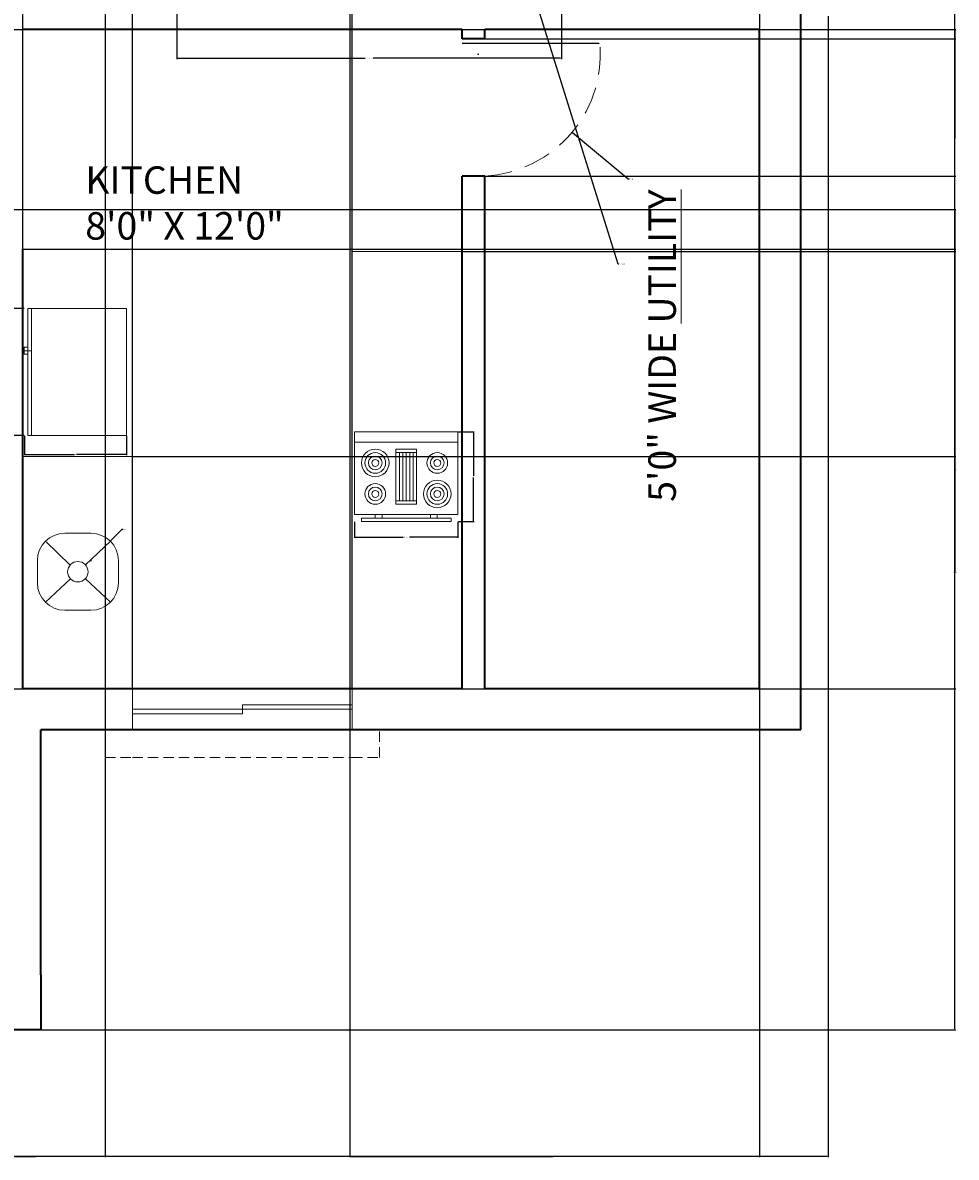
# Model space of a CAD drawing. Units: inches. Extents: x 6662 to 7211, y 5077 to 5683.
# Tile 4 of 9: x 7007 to 7211, y 5077 to 5325. Entities that reach past the tile are written whole.
import ezdxf

# ---------------------------------------------------------------- set-up
doc = ezdxf.new("R2010")
doc.units = ezdxf.units.IN
doc.header["$LTSCALE"] = 3
doc.header["$MEASUREMENT"] = 0
doc.linetypes.add('HIDDEN', pattern=[0.375, 0.25, -0.125])
for name, color, linetype, lineweight in [('A-ANNO-DIMS', 2, 'Continuous', 18), ('A-AREA-IDEN', 7, 'Continuous', 18), ('A-DOOR', 4, 'Continuous', 25), ('A-DOOR-HIDN', 4, 'HIDDEN', 13), ('A-EQPM', 8, 'Continuous', 18), ('A-FLOR-CASE', 8, 'Continuous', 20), ('A-FLOR-CASE-PATT', 241, 'Continuous', 13), ('A-FLOR-FIXT', 8, 'Continuous', 18), ('A-GLAZ', 4, 'Continuous', 18), ('A-GLAZ-OVHD', 4, 'HIDDEN', 13), ('A-WALL', 7, 'Continuous', 35)]:
    doc.layers.add(name, color=color, linetype=linetype, lineweight=lineweight)
doc.styles.get("Standard").update_dxf_attribs({"font": 'arial.ttf'})
doc.dimstyles.get("Standard").update_dxf_attribs({"dimtxt": 0.18, "dimasz": 0.18, "dimexe": 0.18, "dimexo": 0.0625, "dimgap": 0.09, "dimtad": 0, "dimtih": 1, "dimtoh": 1, "dimdec": 4, "dimzin": 0, "dimdsep": 46, "dimtxsty": 'Standard', "dimcen": 0.09, "dimadec": 0, "dimazin": 0, "dimtfac": 1, "dimtdec": 4, "dimtofl": 0, "dimtmove": 0, "dimatfit": 3, "dimfxl": 1, "dimtolj": 1, "dimtzin": 0, "dimarcsym": 0})

# ---------------------------------------------------------------- blocks, each defined once
blk = doc.blocks.new('Range-Oven - 30 in top')
for p, q in [((0, -3), (30, -3)), ((12, -6), (18, -6)), ((13, -20), (13, -6)), ((14, -6), (14, -20)), ((15, -20), (15, -6)), ((16, -6), (16, -20)), ((17, -20), (17, -6)), ((18, -20), (12, -20)), ((6, -24), (6, -25)), ((8, -25), (8, -24)), ((22, -25), (22, -24)), ((24, -24), (24, -25))]:
    blk.add_line(p, q)
for points in [[(0, -24), (0, 0), (30, 0), (30, -24)], [(12, -21), (12, -5), (18, -5), (18, -21)], [(2, -26), (2, -25), (28, -25), (28, -26)]]:
    blk.add_lwpolyline(points, close=True)
for centre, radius in [((6, -9), 4), ((6, -9), 3), ((24, -9), 3), ((6, -9), 2), ((6, -9), 1), ((24, -9), 2), ((24, -9), 1), ((6, -18), 3), ((6, -18), 2), ((24, -18), 4), ((24, -18), 3), ((24, -18), 2), ((6, -18), 1), ((24, -18), 1)]:
    blk.add_circle(centre, radius)
blk = doc.blocks.new('Refrigerator-2 door - 36 in top')
for p, q in [((0, -26.999999), (36, -26.999999)), ((11, -27.999999), (11, -28.999999)), ((12, -26.999999), (12, -28.999999)), ((13, -28.999999), (13, -27.999999)), ((11, -28.999999), (13, -28.999999))]:
    blk.add_line(p, q)
blk.add_lwpolyline([(0, -27.999999), (0, 0), (36, 0), (36, -27.999999)], close=True)
blk = doc.blocks.new('*D28')
at = {"layer": 'A-ANNO-DIMS', "color": 0, "lineweight": -2, "ltscale": 3, "transparency": 16777216}
for p, q in [((7040.57, 5329.37), (7040.57, 5316.65)), ((7124.57, 5329.37), (7124.57, 5316.65)), ((7040.75, 5316.83), (7081.66, 5316.83)), ((7124.39, 5316.83), (7083.47, 5316.83))]:
    blk.add_line(p, q, dxfattribs=at)
at = {"layer": 'A-ANNO-DIMS', "color": 0, "ltscale": 3, "transparency": 16777216}
for points in [[(7040.75, 5316.86), (7040.75, 5316.8), (7040.57, 5316.83)], [(7124.39, 5316.86), (7124.39, 5316.8), (7124.57, 5316.83)]]:
    blk.add_solid(points, dxfattribs=at)
at = {"layer": 'Defpoints', "color": 0, "ltscale": 3, "transparency": 16777216}
for p in [(7040.57, 5329.43), (7124.57, 5329.43), (7040.57, 5316.83)]:
    blk.add_point(p, dxfattribs=at)
at = {"layer": 'A-ANNO-DIMS', "color": 0, "ltscale": 3, "transparency": 16777216, "insert": (7082.57, 5316.83), "char_height": 0.18, "attachment_point": 5}
blk.add_mtext('\\A1;SOFA 84 TYP.', dxfattribs=at)
blk = doc.blocks.new('*D34')
at = {"layer": 'A-ANNO-DIMS', "color": 0, "lineweight": -2, "ltscale": 3, "transparency": 16777216}
for p, q in [((7079.39, 5215.56), (7079.39, 5212.05)), ((7101.96, 5215.56), (7101.96, 5212.05)), ((7079.57, 5212.23), (7089.98, 5212.23)), ((7101.78, 5212.23), (7091.37, 5212.23))]:
    blk.add_line(p, q, dxfattribs=at)
at = {"layer": 'A-ANNO-DIMS', "color": 0, "ltscale": 3, "transparency": 16777216}
for points in [[(7079.57, 5212.26), (7079.57, 5212.2), (7079.39, 5212.23)], [(7101.78, 5212.26), (7101.78, 5212.2), (7101.96, 5212.23)]]:
    blk.add_solid(points, dxfattribs=at)
at = {"layer": 'Defpoints', "color": 0, "ltscale": 3, "transparency": 16777216}
for p in [(7079.39, 5215.62), (7101.96, 5215.62), (7101.96, 5212.23)]:
    blk.add_point(p, dxfattribs=at)
at = {"layer": 'A-ANNO-DIMS', "color": 0, "ltscale": 3, "transparency": 16777216, "insert": (7090.67, 5212.23), "char_height": 0.18, "attachment_point": 5}
blk.add_mtext('\\A1;RANGE 23', dxfattribs=at)
blk = doc.blocks.new('*D35')
at = {"layer": 'A-ANNO-DIMS', "color": 0, "lineweight": -2, "ltscale": 3, "transparency": 16777216}
for p, q in [((7102.02, 5235.18), (7105.53, 5235.18)), ((7105.35, 5235), (7105.35, 5225.58)), ((7105.35, 5215.8), (7105.35, 5225.22)), ((7102.02, 5215.62), (7105.53, 5215.62))]:
    blk.add_line(p, q, dxfattribs=at)
at = {"layer": 'A-ANNO-DIMS', "color": 0, "ltscale": 3, "transparency": 16777216}
for points in [[(7105.32, 5235), (7105.38, 5235), (7105.35, 5235.18)], [(7105.32, 5215.8), (7105.38, 5215.8), (7105.35, 5215.62)]]:
    blk.add_solid(points, dxfattribs=at)
at = {"layer": 'Defpoints', "color": 0, "ltscale": 3, "transparency": 16777216}
for p in [(7101.96, 5235.18), (7105.35, 5235.18), (7101.96, 5215.62)]:
    blk.add_point(p, dxfattribs=at)
at = {"layer": 'A-ANNO-DIMS', "color": 0, "ltscale": 3, "transparency": 16777216, "insert": (7105.35, 5225.4), "char_height": 0.18, "attachment_point": 5}
blk.add_mtext('\\A1;20', dxfattribs=at)
blk = doc.blocks.new('*D36')
at = {"layer": 'A-ANNO-DIMS', "color": 0, "lineweight": -2, "ltscale": 3, "transparency": 16777216}
for p, q in [((7007.15, 5262.16), (7002.88, 5262.16)), ((7003.06, 5261.98), (7003.06, 5248.48)), ((7003.06, 5234.61), (7003.06, 5248.11)), ((7007.15, 5234.43), (7002.88, 5234.43))]:
    blk.add_line(p, q, dxfattribs=at)
at = {"layer": 'A-ANNO-DIMS', "color": 0, "ltscale": 3, "transparency": 16777216}
for points in [[(7003.03, 5261.98), (7003.09, 5261.98), (7003.06, 5262.16)], [(7003.03, 5234.61), (7003.09, 5234.61), (7003.06, 5234.43)]]:
    blk.add_solid(points, dxfattribs=at)
at = {"layer": 'Defpoints', "color": 0, "ltscale": 3, "transparency": 16777216}
for p in [(7007.22, 5262.16), (7003.06, 5234.43), (7007.22, 5234.43)]:
    blk.add_point(p, dxfattribs=at)
at = {"layer": 'A-ANNO-DIMS', "color": 0, "ltscale": 3, "transparency": 16777216, "insert": (7003.06, 5248.29), "char_height": 0.18, "attachment_point": 5}
blk.add_mtext('\\A1;REFRIGERATOR 28', dxfattribs=at)
blk = doc.blocks.new('*D37')
at = {"layer": 'A-ANNO-DIMS', "color": 0, "lineweight": -2, "ltscale": 3, "transparency": 16777216}
for p, q in [((7007.22, 5234.37), (7007.22, 5230.09)), ((7029.56, 5234.37), (7029.56, 5230.09)), ((7007.4, 5230.27), (7018.17, 5230.27)), ((7029.38, 5230.27), (7018.61, 5230.27))]:
    blk.add_line(p, q, dxfattribs=at)
at = {"layer": 'A-ANNO-DIMS', "color": 0, "ltscale": 3, "transparency": 16777216}
for points in [[(7007.4, 5230.3), (7007.4, 5230.24), (7007.22, 5230.27)], [(7029.38, 5230.3), (7029.38, 5230.24), (7029.56, 5230.27)]]:
    blk.add_solid(points, dxfattribs=at)
at = {"layer": 'Defpoints', "color": 0, "ltscale": 3, "transparency": 16777216}
for p in [(7007.22, 5234.43), (7029.56, 5234.43), (7029.56, 5230.27)]:
    blk.add_point(p, dxfattribs=at)
at = {"layer": 'A-ANNO-DIMS', "color": 0, "ltscale": 3, "transparency": 16777216, "insert": (7018.39, 5230.27), "char_height": 0.18, "attachment_point": 5}
blk.add_mtext('\\A1;22', dxfattribs=at)
blk = doc.blocks.new('*D40')
at = {"layer": 'A-ANNO-DIMS', "color": 0, "lineweight": -2, "ltscale": 3, "transparency": 16777216}
for p, q in [((7182.86, 5326.04), (7182.86, 5076.72)), ((6689.86, 5323.04), (6689.86, 5076.72)), ((6690.04, 5076.9), (6936.07, 5076.9)), ((7182.68, 5076.9), (6936.65, 5076.9))]:
    blk.add_line(p, q, dxfattribs=at)
at = {"layer": 'A-ANNO-DIMS', "color": 0, "ltscale": 3, "transparency": 16777216}
for points in [[(6690.04, 5076.93), (6690.04, 5076.87), (6689.86, 5076.9)], [(7182.68, 5076.93), (7182.68, 5076.87), (7182.86, 5076.9)]]:
    blk.add_solid(points, dxfattribs=at)
at = {"layer": 'Defpoints', "color": 0, "ltscale": 3, "transparency": 16777216}
for p in [(7182.86, 5326.1), (6689.86, 5323.1), (7182.86, 5076.9)]:
    blk.add_point(p, dxfattribs=at)
at = {"layer": 'A-ANNO-DIMS', "color": 0, "ltscale": 3, "transparency": 16777216, "insert": (6936.36, 5076.9), "char_height": 0.18, "attachment_point": 5}
blk.add_mtext('\\A1;493', dxfattribs=at)
blk = doc.blocks.new('*D41')
at = {"layer": 'A-ANNO-DIMS', "color": 0, "lineweight": -2, "ltscale": 3, "transparency": 16777216}
for p, q in [((7035.92, 5655.02), (7210.74, 5655.02)), ((7210.56, 5654.84), (7210.56, 5379.99)), ((7210.56, 5104.78), (7210.56, 5379.63)), ((7010.92, 5104.6), (7210.74, 5104.6))]:
    blk.add_line(p, q, dxfattribs=at)
at = {"layer": 'A-ANNO-DIMS', "color": 0, "ltscale": 3, "transparency": 16777216}
for points in [[(7210.53, 5654.84), (7210.59, 5654.84), (7210.56, 5655.02)], [(7210.53, 5104.78), (7210.59, 5104.78), (7210.56, 5104.6)]]:
    blk.add_solid(points, dxfattribs=at)
at = {"layer": 'Defpoints', "color": 0, "ltscale": 3, "transparency": 16777216}
for p in [(7035.86, 5655.02), (7210.56, 5655.02), (7010.86, 5104.6)]:
    blk.add_point(p, dxfattribs=at)
at = {"layer": 'A-ANNO-DIMS', "color": 0, "ltscale": 3, "transparency": 16777216, "insert": (7210.56, 5379.81), "char_height": 0.18, "attachment_point": 5}
blk.add_mtext('\\A1;550.4', dxfattribs=at)
blk = doc.blocks.new('*D67')
at = {"layer": 'A-ANNO-DIMS', "color": 0, "lineweight": -2, "ltscale": 3, "transparency": 16777216}
for p, q in [((6994.86, 5514.54), (6994.86, 5076.72)), ((7024.86, 5514.54), (7024.86, 5076.72)), ((6995.04, 5076.9), (7009.64, 5076.9)), ((7024.68, 5076.9), (7010.08, 5076.9))]:
    blk.add_line(p, q, dxfattribs=at)
at = {"layer": 'A-ANNO-DIMS', "color": 0, "ltscale": 3, "transparency": 16777216}
for points in [[(6995.04, 5076.93), (6995.04, 5076.87), (6994.86, 5076.9)], [(7024.68, 5076.93), (7024.68, 5076.87), (7024.86, 5076.9)]]:
    blk.add_solid(points, dxfattribs=at)
at = {"layer": 'Defpoints', "color": 0, "ltscale": 3, "transparency": 16777216}
for p in [(6994.86, 5514.6), (7024.86, 5514.6), (7024.86, 5076.9)]:
    blk.add_point(p, dxfattribs=at)
at = {"layer": 'A-ANNO-DIMS', "color": 0, "ltscale": 3, "transparency": 16777216, "insert": (7009.86, 5076.9), "char_height": 0.18, "attachment_point": 5}
blk.add_mtext('\\A1;30', dxfattribs=at)
blk = doc.blocks.new('*D69')
at = {"layer": 'A-ANNO-DIMS', "color": 0, "lineweight": -2, "ltscale": 3, "transparency": 16777216}
for p, q in [((7107.92, 5321.1), (7210.74, 5321.1)), ((7210.56, 5320.92), (7210.56, 5306.28)), ((7210.56, 5291.28), (7210.56, 5305.92)), ((7107.92, 5291.1), (7210.74, 5291.1))]:
    blk.add_line(p, q, dxfattribs=at)
at = {"layer": 'A-ANNO-DIMS', "color": 0, "ltscale": 3, "transparency": 16777216}
for points in [[(7210.53, 5320.92), (7210.59, 5320.92), (7210.56, 5321.1)], [(7210.53, 5291.28), (7210.59, 5291.28), (7210.56, 5291.1)]]:
    blk.add_solid(points, dxfattribs=at)
at = {"layer": 'Defpoints', "color": 0, "ltscale": 3, "transparency": 16777216}
for p in [(7107.86, 5321.1), (7210.56, 5321.1), (7107.86, 5291.1)]:
    blk.add_point(p, dxfattribs=at)
at = {"layer": 'A-ANNO-DIMS', "color": 0, "ltscale": 3, "transparency": 16777216, "insert": (7210.56, 5306.1), "char_height": 0.18, "attachment_point": 5}
blk.add_mtext('\\A1;30', dxfattribs=at)
blk = doc.blocks.new('*D74')
at = {"layer": 'A-ANNO-DIMS', "color": 0, "lineweight": -2, "ltscale": 3, "transparency": 16777216}
for p, q in [((7006.86, 5179.16), (7006.86, 5682.9)), ((7007.04, 5682.72), (7018.64, 5682.72)), ((7030.68, 5682.72), (7019.08, 5682.72)), ((7030.86, 5179.16), (7030.86, 5682.9))]:
    blk.add_line(p, q, dxfattribs=at)
at = {"layer": 'A-ANNO-DIMS', "color": 0, "ltscale": 3, "transparency": 16777216}
for points in [[(7007.04, 5682.75), (7007.04, 5682.69), (7006.86, 5682.72)], [(7030.68, 5682.75), (7030.68, 5682.69), (7030.86, 5682.72)]]:
    blk.add_solid(points, dxfattribs=at)
at = {"layer": 'Defpoints', "color": 0, "ltscale": 3, "transparency": 16777216}
for p in [(7030.86, 5682.72), (7006.86, 5179.1), (7030.86, 5179.1)]:
    blk.add_point(p, dxfattribs=at)
at = {"layer": 'A-ANNO-DIMS', "color": 0, "ltscale": 3, "transparency": 16777216, "insert": (7018.86, 5682.72), "char_height": 0.18, "attachment_point": 5}
blk.add_mtext('\\A1;24', dxfattribs=at)
blk = doc.blocks.new('*D75')
at = {"layer": 'A-ANNO-DIMS', "color": 0, "lineweight": -2, "ltscale": 3, "transparency": 16777216}
for p, q in [((7030.86, 5179.16), (7030.86, 5682.9)), ((7031.04, 5682.72), (7054.64, 5682.72)), ((7078.68, 5682.72), (7055.08, 5682.72)), ((7078.86, 5179.16), (7078.86, 5682.9))]:
    blk.add_line(p, q, dxfattribs=at)
at = {"layer": 'A-ANNO-DIMS', "color": 0, "ltscale": 3, "transparency": 16777216}
for points in [[(7031.04, 5682.75), (7031.04, 5682.69), (7030.86, 5682.72)], [(7078.68, 5682.75), (7078.68, 5682.69), (7078.86, 5682.72)]]:
    blk.add_solid(points, dxfattribs=at)
at = {"layer": 'Defpoints', "color": 0, "ltscale": 3, "transparency": 16777216}
for p in [(7078.86, 5682.72), (7030.86, 5179.1), (7078.86, 5179.1)]:
    blk.add_point(p, dxfattribs=at)
at = {"layer": 'A-ANNO-DIMS', "color": 0, "ltscale": 3, "transparency": 16777216, "insert": (7054.86, 5682.72), "char_height": 0.18, "attachment_point": 5}
blk.add_mtext('\\A1;48', dxfattribs=at)
blk = doc.blocks.new('*D78')
at = {"layer": 'A-ANNO-DIMS', "color": 0, "lineweight": -2, "ltscale": 3, "transparency": 16777216}
for p, q in [((7001.92, 5323.1), (7210.74, 5323.1)), ((7210.56, 5322.92), (7210.56, 5299.28)), ((7210.56, 5275.28), (7210.56, 5298.92)), ((7006.92, 5275.1), (7210.74, 5275.1))]:
    blk.add_line(p, q, dxfattribs=at)
at = {"layer": 'A-ANNO-DIMS', "color": 0, "ltscale": 3, "transparency": 16777216}
for points in [[(7210.53, 5322.92), (7210.59, 5322.92), (7210.56, 5323.1)], [(7210.53, 5275.28), (7210.59, 5275.28), (7210.56, 5275.1)]]:
    blk.add_solid(points, dxfattribs=at)
at = {"layer": 'Defpoints', "color": 0, "ltscale": 3, "transparency": 16777216}
for p in [(7001.86, 5323.1), (7210.56, 5323.1), (7006.86, 5275.1)]:
    blk.add_point(p, dxfattribs=at)
at = {"layer": 'A-ANNO-DIMS', "color": 0, "ltscale": 3, "transparency": 16777216, "insert": (7210.56, 5299.1), "char_height": 0.18, "attachment_point": 5}
blk.add_mtext('\\A1;48', dxfattribs=at)
blk = doc.blocks.new('*D81')
at = {"layer": 'A-ANNO-DIMS', "color": 0, "lineweight": -2, "ltscale": 3, "transparency": 16777216}
for p, q in [((7078.36, 5473.54), (7078.36, 5076.72)), ((7167.86, 5473.54), (7167.86, 5076.72)), ((7078.54, 5076.9), (7122.78, 5076.9)), ((7167.68, 5076.9), (7123.43, 5076.9))]:
    blk.add_line(p, q, dxfattribs=at)
at = {"layer": 'A-ANNO-DIMS', "color": 0, "ltscale": 3, "transparency": 16777216}
for points in [[(7078.54, 5076.93), (7078.54, 5076.87), (7078.36, 5076.9)], [(7167.68, 5076.93), (7167.68, 5076.87), (7167.86, 5076.9)]]:
    blk.add_solid(points, dxfattribs=at)
at = {"layer": 'Defpoints', "color": 0, "ltscale": 3, "transparency": 16777216}
for p in [(7078.36, 5473.6), (7167.86, 5473.6), (7167.86, 5076.9)]:
    blk.add_point(p, dxfattribs=at)
at = {"layer": 'A-ANNO-DIMS', "color": 0, "ltscale": 3, "transparency": 16777216, "insert": (7123.11, 5076.9), "char_height": 0.18, "attachment_point": 5}
blk.add_mtext('\\A1;89.5', dxfattribs=at)
blk = doc.blocks.new('*D83')
at = {"layer": 'A-ANNO-DIMS', "color": 0, "lineweight": -2, "ltscale": 3, "transparency": 16777216}
for p, q in [((6845.92, 5283.8), (7210.74, 5283.8)), ((7210.56, 5283.62), (7210.56, 5231.63)), ((7210.56, 5179.28), (7210.56, 5231.27)), ((6845.92, 5179.1), (7210.74, 5179.1))]:
    blk.add_line(p, q, dxfattribs=at)
at = {"layer": 'A-ANNO-DIMS', "color": 0, "ltscale": 3, "transparency": 16777216}
for points in [[(7210.53, 5283.62), (7210.59, 5283.62), (7210.56, 5283.8)], [(7210.53, 5179.28), (7210.59, 5179.28), (7210.56, 5179.1)]]:
    blk.add_solid(points, dxfattribs=at)
at = {"layer": 'Defpoints', "color": 0, "ltscale": 3, "transparency": 16777216}
for p in [(6845.86, 5283.8), (7210.56, 5283.8), (6845.86, 5179.1)]:
    blk.add_point(p, dxfattribs=at)
at = {"layer": 'A-ANNO-DIMS', "color": 0, "ltscale": 3, "transparency": 16777216, "insert": (7210.56, 5231.45), "char_height": 0.18, "attachment_point": 5}
blk.add_mtext('\\A1;104.7', dxfattribs=at)
blk = doc.blocks.new('*D85')
at = {"layer": 'A-ANNO-DIMS', "color": 0, "lineweight": -2, "ltscale": 3, "transparency": 16777216}
for p, q in [((7030.92, 5229.86), (7210.74, 5229.86)), ((7210.56, 5229.68), (7210.56, 5204.66)), ((7210.56, 5179.28), (7210.56, 5204.3)), ((7030.92, 5179.1), (7210.74, 5179.1))]:
    blk.add_line(p, q, dxfattribs=at)
at = {"layer": 'A-ANNO-DIMS', "color": 0, "ltscale": 3, "transparency": 16777216}
for points in [[(7210.53, 5229.68), (7210.59, 5229.68), (7210.56, 5229.86)], [(7210.53, 5179.28), (7210.59, 5179.28), (7210.56, 5179.1)]]:
    blk.add_solid(points, dxfattribs=at)
at = {"layer": 'Defpoints', "color": 0, "ltscale": 3, "transparency": 16777216}
for p in [(7030.86, 5229.86), (7210.56, 5229.86), (7030.86, 5179.1)]:
    blk.add_point(p, dxfattribs=at)
at = {"layer": 'A-ANNO-DIMS', "color": 0, "ltscale": 3, "transparency": 16777216, "insert": (7210.56, 5204.48), "char_height": 0.18, "attachment_point": 5}
blk.add_mtext('\\A1;50.76', dxfattribs=at)
blk = doc.blocks.new('*D86')
at = {"layer": 'A-ANNO-DIMS', "color": 0, "lineweight": -2, "ltscale": 3, "transparency": 16777216}
for p, q in [((7102.92, 5274.62), (7210.74, 5274.62)), ((7210.56, 5274.44), (7210.56, 5227.04)), ((7210.56, 5179.28), (7210.56, 5226.68)), ((7102.92, 5179.1), (7210.74, 5179.1))]:
    blk.add_line(p, q, dxfattribs=at)
at = {"layer": 'A-ANNO-DIMS', "color": 0, "ltscale": 3, "transparency": 16777216}
for points in [[(7210.53, 5274.44), (7210.59, 5274.44), (7210.56, 5274.62)], [(7210.53, 5179.28), (7210.59, 5179.28), (7210.56, 5179.1)]]:
    blk.add_solid(points, dxfattribs=at)
at = {"layer": 'Defpoints', "color": 0, "ltscale": 3, "transparency": 16777216}
for p in [(7102.86, 5274.62), (7210.56, 5274.62), (7102.86, 5179.1)]:
    blk.add_point(p, dxfattribs=at)
at = {"layer": 'A-ANNO-DIMS', "color": 0, "ltscale": 3, "transparency": 16777216, "insert": (7210.56, 5226.86), "char_height": 0.18, "attachment_point": 5}
blk.add_mtext('\\A1;95.53', dxfattribs=at)
blk = doc.blocks.new('*D94')
at = {"layer": 'A-ANNO-DIMS', "color": 0, "lineweight": -2, "ltscale": 3, "transparency": 16777216}
for p, q in [((7106.33, 5317.71), (7106.51, 5317.71)), ((7106.42, 5317.62), (7106.42, 5317.8)), ((7139.18, 5290.41), (7127.03, 5300.53)), ((7139.36, 5290.41), (7139.18, 5290.41))]:
    blk.add_line(p, q, dxfattribs=at)
at = {"layer": 'A-ANNO-DIMS', "color": 0, "ltscale": 3, "transparency": 16777216}
blk.add_solid([(7127.05, 5300.56), (7127.02, 5300.51), (7126.9, 5300.65)], dxfattribs=at)
at = {"layer": 'Defpoints', "color": 0, "ltscale": 3, "transparency": 16777216}
for p in [(7106.42, 5317.71), (7126.9, 5300.65)]:
    blk.add_point(p, dxfattribs=at)
at = {"layer": 'A-ANNO-DIMS', "color": 0, "ltscale": 3, "transparency": 16777216, "insert": (7139.84, 5290.41), "char_height": 0.18, "attachment_point": 5}
blk.add_mtext('\\A1;R26.65', dxfattribs=at)
blk = doc.blocks.new('*D99')
at = {"layer": 'A-ANNO-DIMS', "color": 0, "lineweight": -2, "ltscale": 3, "transparency": 16777216}
for p, q in [((7028.55, 5213.86), (7026.14, 5211.44)), ((7028.73, 5213.86), (7028.55, 5213.86)), ((7021.68, 5207.07), (7021.86, 5207.07)), ((7021.77, 5206.98), (7021.77, 5207.16))]:
    blk.add_line(p, q, dxfattribs=at)
at = {"layer": 'A-ANNO-DIMS', "color": 0, "ltscale": 3, "transparency": 16777216}
blk.add_solid([(7026.12, 5211.46), (7026.16, 5211.42), (7026.01, 5211.31)], dxfattribs=at)
at = {"layer": 'Defpoints', "color": 0, "ltscale": 3, "transparency": 16777216}
for p in [(7026.01, 5211.31), (7021.77, 5207.07)]:
    blk.add_point(p, dxfattribs=at)
at = {"layer": 'A-ANNO-DIMS', "color": 0, "ltscale": 3, "transparency": 16777216, "insert": (7029.17, 5213.86), "char_height": 0.18, "attachment_point": 5}
blk.add_mtext('\\A1;4X R6', dxfattribs=at)
blk = doc.blocks.new('*D101')
at = {"layer": 'A-ANNO-DIMS', "color": 0, "lineweight": -2, "ltscale": 3, "transparency": 16777216}
for p, q in [((7082.48, 5446.35), (7082.66, 5446.35)), ((7082.57, 5446.26), (7082.57, 5446.44)), ((7136.97, 5271.83), (7116.62, 5337.1)), ((7137.15, 5271.83), (7136.97, 5271.83))]:
    blk.add_line(p, q, dxfattribs=at)
at = {"layer": 'A-ANNO-DIMS', "color": 0, "ltscale": 3, "transparency": 16777216}
blk.add_solid([(7116.65, 5337.11), (7116.6, 5337.09), (7116.57, 5337.27)], dxfattribs=at)
at = {"layer": 'Defpoints', "color": 0, "ltscale": 3, "transparency": 16777216}
for p in [(7082.57, 5446.35), (7116.57, 5337.27)]:
    blk.add_point(p, dxfattribs=at)
at = {"layer": 'A-ANNO-DIMS', "color": 0, "ltscale": 3, "transparency": 16777216, "insert": (7137.9, 5271.83), "char_height": 0.18, "attachment_point": 5}
blk.add_mtext('\\A1;2X R114.25', dxfattribs=at)

msp = doc.modelspace()

# ---------------------------------------------------------------- hatches: boundary and pattern name
at = {"layer": 'A-FLOR-CASE-PATT'}
h = msp.add_hatch(dxfattribs=at)
h.set_pattern_fill('ANSI31', color=256)
h.paths.add_polyline_path([(6869.8579, 5283.7981), (6845.8579, 5283.7981), (6845.8579, 5229.4653), (6847.018, 5229.7817, -0.54116316), (6849.0925, 5228.1371), (6849.7129, 5228.234, -0.50821327), (6851.018, 5227.2817), (6851.018, 5226.7817), (6855.018, 5227.2817), (6855.018, 5225.7817), (6851.018, 5225.2817), (6851.018, 5217.7817), (6851.018, 5210.2817), (6855.018, 5209.7817), (6855.018, 5208.2817), (6851.018, 5208.7817), (6851.018, 5208.2817, -0.41421356), (6850.018, 5207.2817), (6849.0925, 5207.4263, -0.50580924), (6847.1872, 5205.7355), (6845.8579, 5206.0981), (6845.8579, 5179.0979), (6869.8579, 5179.0979)])
h.paths.add_polyline_path([(7167.8579, 5497.5979), (7143.8579, 5497.5979), (7078.3579, 5497.5979), (7078.3579, 5473.5979), (7163.8579, 5473.5979), (7167.8579, 5473.5979)])
h.paths.add_polyline_path([(6825.9016, 5497.5979), (6725.8579, 5497.5979), (6725.8579, 5473.5979), (6825.9016, 5473.5979)])
h.paths.add_polyline_path([(6796.6359, 5485.2095), (6797.1359, 5489.2095), (6806.1359, 5489.2095), (6815.1359, 5489.2095), (6815.6359, 5485.2095), (6814.1359, 5485.2095), (6813.6359, 5489.2095), (6806.1359, 5489.2095), (6798.6359, 5489.2095), (6798.1359, 5485.2095)], flags=16)

# ---------------------------------------------------------------- linework, layer by layer
at = {"layer": 'A-DOOR'}
for p, q in [((7102.8579, 5321.0979), (7132.8579, 5321.0979)), ((7102.8579, 5320.0979), (7132.8579, 5320.0979))]:
    msp.add_line(p, q, dxfattribs=at)
at = {"layer": 'A-DOOR-HIDN', "ltscale": 8}
msp.add_arc((7106.4217, 5317.7114), 26.6522, 273.088813, 7.300045, dxfattribs=at)
at = {"layer": 'A-FLOR-CASE'}
for p, q in [((7078.8579, 5170.0979), (7078.8579, 5274.6249)), ((7078.8579, 5274.6249), (7102.8579, 5274.6249)), ((7030.8579, 5229.858), (7006.8579, 5229.858)), ((7030.8579, 5170.0979), (7030.8579, 5229.858))]:
    msp.add_line(p, q, dxfattribs=at)
at = {"layer": 'A-FLOR-FIXT'}
for p, q in [((7017.2293, 5206.1192), (7011.8218, 5211.3111)), ((7026.0094, 5211.3111), (7020.5476, 5206.1791)), ((7011.8218, 5197.9802), (7017.2836, 5203.1122)), ((7026.0094, 5197.9802), (7020.5476, 5203.1122))]:
    msp.add_line(p, q, dxfattribs=at)
msp.add_lwpolyline([(7016.0644, 5213.0684), (7021.7668, 5213.0684, -0.41421356), (7027.7668, 5207.0684), (7027.7668, 5202.2228, -0.41421356), (7021.7668, 5196.2228), (7016.0644, 5196.2228, -0.41421356), (7010.0644, 5202.2228), (7010.0644, 5207.0684, -0.41421356)], format="xyb", close=True, dxfattribs=at)
msp.add_circle((7018.9156, 5204.6456), 2.2394, dxfattribs=at)
at = {"layer": 'A-GLAZ'}
for p, q in [((7030.8579, 5170.0979), (7030.8579, 5179.0979)), ((7078.8579, 5170.0979), (7078.8579, 5179.0979)), ((7078.8579, 5174.5979), (7030.8579, 5174.5979)), ((7054.8579, 5173.5979), (7030.8579, 5173.5979)), ((7078.8579, 5175.5979), (7054.8579, 5175.5979)), ((7054.8579, 5173.5979), (7054.8579, 5175.5979))]:
    msp.add_line(p, q, dxfattribs=at)
at = {"layer": 'A-GLAZ-OVHD', "ltscale": 3}
for p, q in [((7030.8579, 5170.0979), (7024.8579, 5170.0979)), ((7024.8579, 5170.0979), (7024.8579, 5164.0979)), ((7084.8579, 5164.0979), (7084.8579, 5170.0979)), ((7024.8579, 5164.0979), (7030.8579, 5164.0979)), ((7030.8579, 5164.0979), (7078.8579, 5164.0979)), ((7078.8579, 5164.0979), (7084.8579, 5164.0979))]:
    msp.add_line(p, q, dxfattribs=at)
at = {"layer": 'A-WALL'}
for p, q in [((7176.8579, 5170.0979), (7176.8579, 5398.3479)), ((7102.8579, 5323.0979), (7006.8579, 5323.0979)), ((7102.8579, 5323.0979), (7010.8579, 5323.0979)), ((7102.8579, 5321.0979), (7102.8579, 5323.0979)), ((7167.8579, 5323.0979), (7107.8579, 5323.0979)), ((7107.8579, 5321.0979), (7107.8579, 5323.0979)), ((7167.8579, 5179.0979), (7167.8579, 5323.0979)), ((7107.8579, 5321.0979), (7102.8579, 5321.0979)), ((7102.8579, 5179.0979), (7102.8579, 5291.0979)), ((7107.8579, 5291.0979), (7102.8579, 5291.0979)), ((7107.8579, 5179.0979), (7107.8579, 5291.0979)), ((7006.8579, 5179.0979), (7006.8579, 5275.0979)), ((7102.8579, 5179.0979), (7006.8579, 5179.0979)), ((7167.8579, 5179.0979), (7107.8579, 5179.0979)), ((7167.8579, 5179.0979), (7112.8579, 5179.0979)), ((7176.8579, 5170.0979), (7010.8579, 5170.0979)), ((7010.8579, 5116.5979), (7010.8579, 5170.0979)), ((7010.8579, 5116.5979), (7010.8579, 5104.5979)), ((7010.8579, 5104.5979), (7001.8579, 5104.5979))]:
    msp.add_line(p, q, dxfattribs=at)

# ---------------------------------------------------------------- block references
at = {"layer": 'A-EQPM', "xscale": 0.7703791697346855, "yscale": 0.7703791697346855, "zscale": 0.7703791697346855, "rotation": 270}
msp.add_blockref('Refrigerator-2 door - 36 in top', (7029.5572, 5262.1612), dxfattribs=at)
at = {"layer": 'A-EQPM', "xscale": 0.7524760752180227, "yscale": 0.7524760752180227, "zscale": 0.7524760752180227}
msp.add_blockref('Range-Oven - 30 in top', (7079.3867, 5235.1845), dxfattribs=at)

# ---------------------------------------------------------------- texts
at = {"layer": 'A-AREA-IDEN', "ltscale": 3, "insert": (7020.5344, 5293.2128), "char_height": 6, "attachment_point": 1}
msp.add_mtext_dynamic_manual_height_columns('KITCHEN\\P8\'0" X 12\'0"', width=381.547883, gutter_width=1, heights=[0], dxfattribs=at)
at = {"layer": 'A-AREA-IDEN', "ltscale": 3, "insert": (7143.5787, 5219.9259), "char_height": 6, "attachment_point": 1, "rotation": 90}
msp.add_mtext_dynamic_manual_height_columns('5\'0" WIDE {\\LUTILITY}', width=381.547883, gutter_width=1, heights=[0], dxfattribs=at)

# ---------------------------------------------------------------- dimensions: what is measured, and where the dimension line sits
at = {"layer": 'A-ANNO-DIMS', "ltscale": 3}
for base, p1, p2, override, picture, middle in [((7030.8579, 5682.7209), (7006.8579, 5179.0979), (7030.8579, 5179.0979), {"dimdec": 0, "dimlfac": 1, "dimrnd": 0, "dimzin": 0, "dimdsep": 46, "dimlunit": 2}, '*D74', (7018.8579, 5682.7209)), ((7078.8579, 5682.7209), (7030.8579, 5179.0979), (7078.8579, 5179.0979), {"dimdec": 0, "dimlfac": 1, "dimrnd": 0, "dimzin": 0, "dimdsep": 46, "dimlunit": 2}, '*D75', (7054.8579, 5682.7209)), ((7024.8579, 5076.8979), (6994.8579, 5514.5979), (7024.8579, 5514.5979), {"dimdec": 0, "dimlfac": 1, "dimrnd": 0, "dimzin": 0, "dimdsep": 46, "dimlunit": 2}, '*D67', (7009.8579, 5076.8979)), ((7167.8579, 5076.8979), (7078.3579, 5473.5979), (7167.8579, 5473.5979), {"dimdec": 1, "dimlfac": 1, "dimrnd": 0, "dimzin": 0, "dimdsep": 46, "dimlunit": 2}, '*D81', (7123.1079, 5076.8979)), ((7182.8579, 5076.8979), (6689.8579, 5323.0979), (7182.8579, 5326.0979), {"dimdec": 0, "dimlfac": 1, "dimrnd": 0, "dimzin": 0, "dimdsep": 46, "dimlunit": 2}, '*D40', (6936.3579, 5076.8979)), ((7029.5572, 5230.2675), (7007.2162, 5234.4275), (7029.5572, 5234.4275), {"dimdec": 0, "dimlfac": 1, "dimrnd": 0, "dimzin": 0, "dimdsep": 46, "dimlunit": 2}, '*D37', (7018.3867, 5230.2675))]:
    dim = msp.add_linear_dim(base=base, p1=p1, p2=p2, dimstyle='Standard', override=override, dxfattribs=at)
    dim.commit()
    dim.dimension.update_dxf_attribs({"geometry": picture, "text_midpoint": middle})
for base, p1, p2, override, picture, middle in [((7210.5579, 5655.0209), (7010.8579, 5104.5979), (7035.8579, 5655.0209), {"dimdec": 1, "dimlfac": 1, "dimrnd": 0, "dimzin": 0, "dimdsep": 46, "dimlunit": 2}, '*D41', (7210.5579, 5379.8094)), ((7210.5579, 5323.0979), (7006.8579, 5275.0979), (7001.8579, 5323.0979), {"dimdec": 0, "dimlfac": 1, "dimrnd": 0, "dimzin": 0, "dimdsep": 46, "dimlunit": 2}, '*D78', (7210.5579, 5299.0979)), ((7210.5579, 5321.0979), (7107.8579, 5291.0979), (7107.8579, 5321.0979), {"dimdec": 0, "dimlfac": 1, "dimrnd": 0, "dimzin": 0, "dimdsep": 46, "dimlunit": 2}, '*D69', (7210.5579, 5306.0979)), ((7210.5579, 5283.7981), (6845.8579, 5179.0979), (6845.8579, 5283.7981), {"dimdec": 1, "dimlfac": 1, "dimrnd": 0, "dimzin": 0, "dimdsep": 46, "dimlunit": 2}, '*D83', (7210.5579, 5231.448)), ((7210.5579, 5274.6249), (7102.8579, 5179.0979), (7102.8579, 5274.6249), {"dimdec": 2, "dimlfac": 1, "dimrnd": 0, "dimzin": 0, "dimdsep": 46, "dimlunit": 2}, '*D86', (7210.5579, 5226.8614)), ((7105.3472, 5235.1845), (7101.961, 5215.6201), (7101.961, 5235.1845), {"dimdec": 0, "dimlfac": 1, "dimrnd": 0, "dimzin": 0, "dimdsep": 46, "dimlunit": 2}, '*D35', (7105.3472, 5225.4023)), ((7210.5579, 5229.858), (7030.8579, 5179.0979), (7030.8579, 5229.858), {"dimdec": 2, "dimlfac": 1, "dimrnd": 0, "dimzin": 0, "dimdsep": 46, "dimlunit": 2}, '*D85', (7210.5579, 5204.4779))]:
    dim = msp.add_linear_dim(base=base, p1=p1, p2=p2, angle=90, dimstyle='Standard', override=override, dxfattribs=at)
    dim.commit()
    dim.dimension.update_dxf_attribs({"geometry": picture, "text_midpoint": middle})
for center, mpoint, text, override, picture, middle in [((7082.5693, 5446.3479), (7116.5707, 5337.2747), '2X <>', {"dimdec": 2, "dimlfac": 1, "dimrnd": 0, "dimzin": 0, "dimdsep": 46, "dimlunit": 2}, '*D101', (7137.8968, 5271.8308)), ((7021.7668, 5207.0684), (7026.0092, 5211.3112), '4X <>', {"dimdec": 0, "dimlfac": 1, "dimrnd": 0, "dimzin": 0, "dimdsep": 46, "dimlunit": 2}, '*D99', (7029.1668, 5213.8569))]:
    dim = msp.add_radius_dim(center=center, mpoint=mpoint, text=text, dimstyle='Standard', override=override, dxfattribs=at)
    dim.commit()
    dim.dimension.update_dxf_attribs({"geometry": picture, "text_midpoint": middle, "dimtype": 164})
for base, p1, p2, angle, text, picture, middle in [((7040.5693, 5316.8313), (7124.5694, 5329.4313), (7040.5693, 5329.4313), 180, 'SOFA <> TYP.', '*D28', (7082.5693, 5316.8313)), ((7003.0561, 5234.4275), (7007.2162, 5262.1612), (7007.2162, 5234.4275), 270, 'REFRIGERATOR <>', '*D36', (7003.0561, 5248.2944))]:
    dim = msp.add_linear_dim(base=base, p1=p1, p2=p2, angle=angle, text=text, dimstyle='Standard', override={"dimdec": 0, "dimlfac": 1, "dimrnd": 0, "dimzin": 0, "dimdsep": 46, "dimlunit": 2}, dxfattribs=at)
    dim.commit()
    dim.dimension.update_dxf_attribs({"geometry": picture, "text_midpoint": middle})
dim = msp.add_radius_dim(center=(7106.4217, 5317.7114), mpoint=(7126.8963, 5300.6488), dimstyle='Standard', override={"dimdec": 2, "dimlfac": 1, "dimrnd": 0, "dimzin": 0, "dimdsep": 46, "dimlunit": 2}, dxfattribs=at)
dim.commit()
dim.dimension.update_dxf_attribs({"geometry": '*D94', "text_midpoint": (7139.8415, 5290.4112), "dimtype": 164})
dim = msp.add_linear_dim(base=(7101.961, 5212.234), p1=(7079.3867, 5215.6201), p2=(7101.961, 5215.6201), text='RANGE <>', dimstyle='Standard', override={"dimdec": 0, "dimlfac": 1, "dimrnd": 0, "dimzin": 0, "dimdsep": 46, "dimlunit": 2}, dxfattribs=at)
dim.commit()
dim.dimension.update_dxf_attribs({"geometry": '*D34', "text_midpoint": (7090.6739, 5212.234)})

doc.saveas('drawing.dxf')
